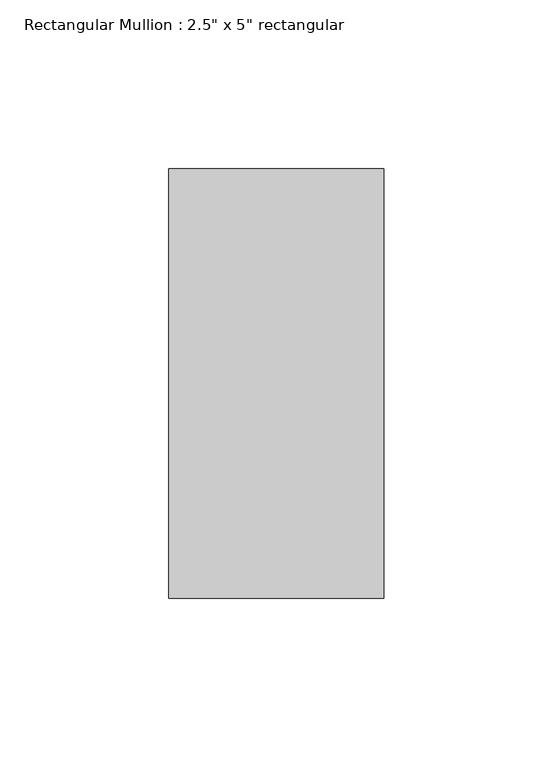
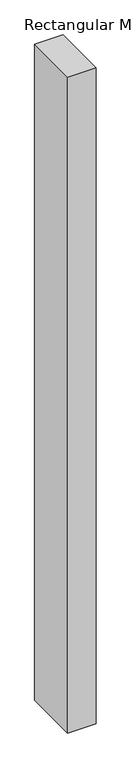
"""IFC4 building model written with IfcOpenShell, lengths in millimetres: member geometry."""

from ifc_helpers import new_model, si_unit, frame, origin, place, context, project, spatial, polyline, outline, extrude, source, transform, mapped, element, save


def member_ed313243(model_context):
    return source(origin(), model_context, "Body", "SweptSolid", [
        extrude(outline(polyline([(0.0, 63.5), (0.0, -63.5), (-63.5, -63.5), (-63.5, 63.5), (0.0, 63.5)])), frame((0.0, 0.0, -1544.0388529), z_axis=(0.0, 0.0, 1.0), x_axis=(1.0, 0.0, 0.0)), (0.0, 0.0, 1.0), 1544.0388529),
    ])


if __name__ == "__main__":
    model = new_model("IFC4")
    model_context = context("Model", 3, world=origin())
    ifc_project = project(units=[si_unit("LENGTHUNIT", "METRE", prefix="MILLI")], contexts=[model_context])
    site = spatial("IfcSite", under=ifc_project)
    building = spatial("IfcBuilding", under=site)
    placement = place(None, origin())
    member_shape = member_ed313243(model_context)
    element("IfcMember", 1, ObjectType="Rectangular Mullion : 2.5\" x 5\" rectangular", at=placement, inside=building, context=model_context, shape_type="MappedRepresentation", body=[
        mapped(member_shape, transform((0.0, 0.0, 0.0), x_axis=(1.0, 0.0, 0.0), y_axis=(0.0, 1.0, 0.0), z_axis=(0.0, 0.0, 1.0))),
    ])
    save(model, "model.ifc")

# Revit data of these elements
# Type "Rectangular Mullion : 2.5\" x 5\" rectangular"
#   built-in parameter 1007304 = 0.416667 (stored number, unit not read)
#   built-in parameter 1007301 = 0.104167 (stored number, unit not read)
#   built-in parameter 1007300 = 0.104167 (stored number, unit not read)
# Element 1 (IfcMember, "Rectangular Mullion : 2.5\" x 5\" rectangular")
#   Materials on its faces: "Aluminum"
# Materials
#   "Aluminum": class "Metal", colour RGB 247 247 247, transparency 0, Description = "Aluminum 6061", Cost = 0
